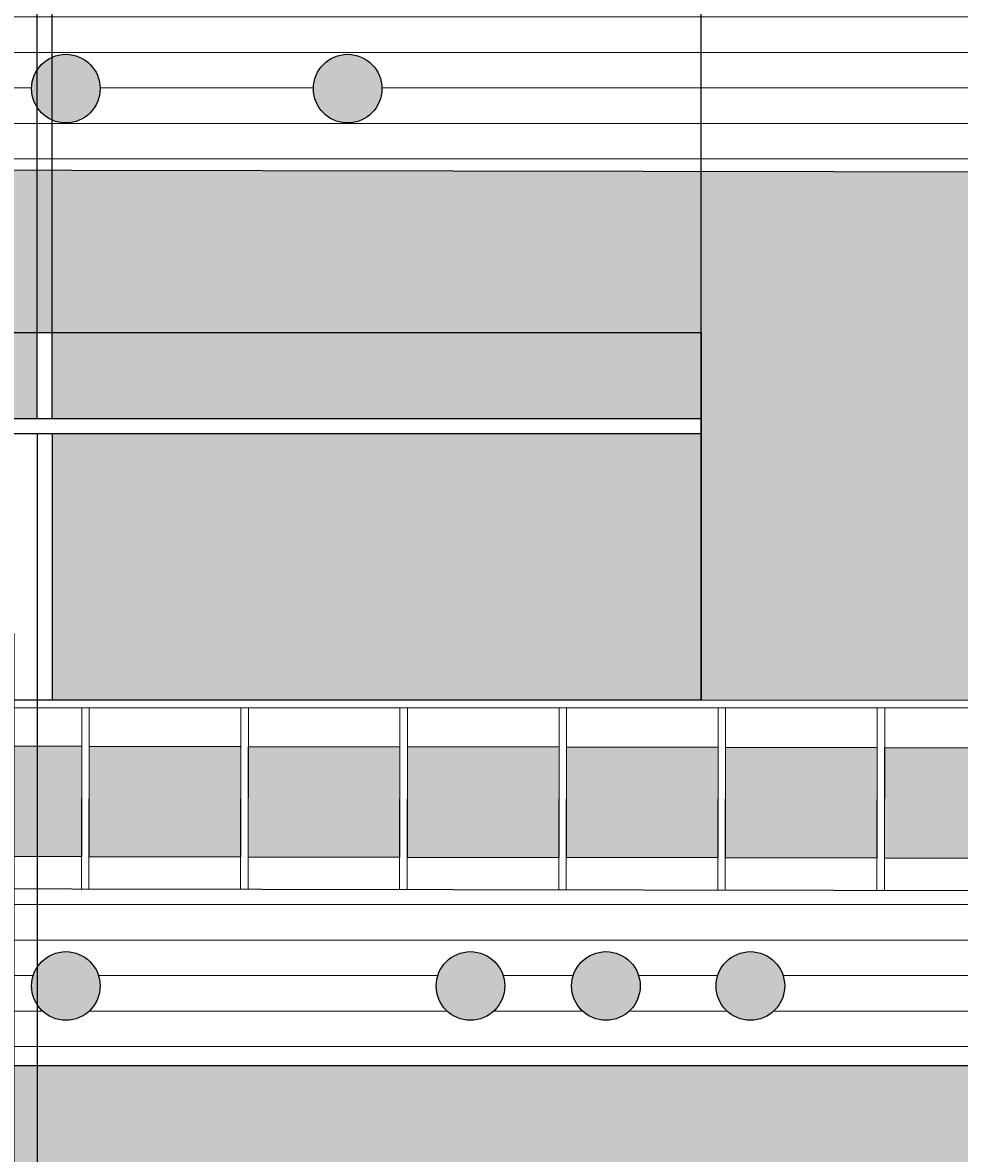
# Model space of a CAD drawing. Units: inches. Extents: x 36 to 594, y 79 to 831.
# Tile 10 of 30: x 265 to 390, y 294 to 446. Entities that reach past the tile are written whole.
import ezdxf

# ---------------------------------------------------------------- set-up
doc = ezdxf.new("R2010")
doc.units = ezdxf.units.IN
doc.header["$MEASUREMENT"] = 0
for name, color, linetype, lineweight in [('A-ANNO-DIMS', 2, 'Continuous', 18), ('A-ELEV', 7, 'Continuous', 25), ('A-ELEV-PATT', 8, 'Continuous', 13), ('A-GLAZ', 4, 'Continuous', 18)]:
    doc.layers.add(name, color=color, linetype=linetype, lineweight=lineweight)
doc.styles.get("Standard").update_dxf_attribs({"font": 'arial.ttf'})
doc.dimstyles.get("Standard").update_dxf_attribs({"dimtxt": 0.8125, "dimasz": 0.18, "dimexe": 0.18, "dimexo": 0.0625, "dimgap": 0.09, "dimtad": 0, "dimtih": 1, "dimtoh": 1, "dimdec": 4, "dimzin": 0, "dimdsep": 46, "dimlunit": 4, "dimtxsty": 'Standard', "dimcen": 0.09, "dimadec": 0, "dimazin": 0, "dimtfac": 1, "dimtdec": 4, "dimtofl": 0, "dimtmove": 0, "dimatfit": 3, "dimfxl": 1, "dimtolj": 1, "dimtzin": 0, "dimarcsym": 0})

# ---------------------------------------------------------------- blocks, each defined once
blk = doc.blocks.new('GLAZ-PANEL')
blk.add_lwpolyline([(0, 14.77), (20.28, 14.77), (20.28, 0), (0, 0)], close=True)
blk = doc.blocks.new('*D28')
at = {"layer": 'A-ANNO-DIMS', "color": 0, "lineweight": -2, "transparency": 16777216}
for p, q in [((269.3, 796.05), (37.49, 796.05)), ((37.67, 795.87), (37.67, 455.63)), ((37.67, 114.39), (37.67, 454.62)), ((94.8, 114.21), (37.49, 114.21))]:
    blk.add_line(p, q, dxfattribs=at)
at = {"layer": 'A-ANNO-DIMS', "color": 0, "transparency": 16777216}
for points in [[(37.64, 795.87), (37.7, 795.87), (37.67, 796.05)], [(37.64, 114.39), (37.7, 114.39), (37.67, 114.21)]]:
    blk.add_solid(points, dxfattribs=at)
at = {"layer": 'Defpoints', "color": 0, "transparency": 16777216}
for p in [(37.67, 796.05), (269.36, 796.05), (94.87, 114.21)]:
    blk.add_point(p, dxfattribs=at)
at = {"layer": 'A-ANNO-DIMS', "color": 0, "transparency": 16777216, "insert": (37.67, 455.13), "char_height": 0.812, "attachment_point": 5}
blk.add_mtext('\\A1;681.8', dxfattribs=at)
blk = doc.blocks.new('*D59')
at = {"layer": 'A-ANNO-DIMS', "color": 0, "lineweight": -2, "transparency": 16777216}
for p, q in [((355.86, 355.15), (355.86, 830.73)), ((356.04, 830.55), (388.74, 830.55)), ((424.37, 830.55), (391.67, 830.55)), ((424.55, 355.15), (424.55, 830.73))]:
    blk.add_line(p, q, dxfattribs=at)
at = {"layer": 'A-ANNO-DIMS', "color": 0, "transparency": 16777216}
for points in [[(356.04, 830.58), (356.04, 830.52), (355.86, 830.55)], [(424.37, 830.58), (424.37, 830.52), (424.55, 830.55)]]:
    blk.add_solid(points, dxfattribs=at)
at = {"layer": 'Defpoints', "color": 0, "transparency": 16777216}
for p in [(424.55, 830.55), (355.86, 355.08), (424.55, 355.08)]:
    blk.add_point(p, dxfattribs=at)
at = {"layer": 'A-ANNO-DIMS', "color": 0, "transparency": 16777216, "insert": (390.2, 830.55), "char_height": 0.812, "attachment_point": 5}
blk.add_mtext('\\A1;68.69', dxfattribs=at)
blk = doc.blocks.new('*D105')
at = {"layer": 'A-ANNO-DIMS', "color": 0, "lineweight": -2, "transparency": 16777216}
for p, q in [((241.36, 404.34), (241.36, 830.73)), ((241.54, 830.55), (252.42, 830.55)), ((266.86, 830.55), (255.98, 830.55)), ((267.04, 404.34), (267.04, 830.73))]:
    blk.add_line(p, q, dxfattribs=at)
at = {"layer": 'A-ANNO-DIMS', "color": 0, "transparency": 16777216}
for points in [[(241.54, 830.58), (241.54, 830.52), (241.36, 830.55)], [(266.86, 830.58), (266.86, 830.52), (267.04, 830.55)]]:
    blk.add_solid(points, dxfattribs=at)
at = {"layer": 'Defpoints', "color": 0, "transparency": 16777216}
for p in [(267.04, 830.55), (241.36, 404.27), (267.04, 404.27)]:
    blk.add_point(p, dxfattribs=at)
at = {"layer": 'A-ANNO-DIMS', "color": 0, "transparency": 16777216, "insert": (254.2, 830.55), "char_height": 0.812, "attachment_point": 5}
blk.add_mtext('\\A1;25.684', dxfattribs=at)
blk = doc.blocks.new('*D106')
at = {"layer": 'A-ANNO-DIMS', "color": 0, "lineweight": -2, "transparency": 16777216}
for p, q in [((267.04, 404.34), (267.04, 830.73)), ((267.22, 830.55), (267.68, 830.55)), ((268.86, 830.55), (268.4, 830.55)), ((269.04, 404.34), (269.04, 830.73))]:
    blk.add_line(p, q, dxfattribs=at)
at = {"layer": 'A-ANNO-DIMS', "color": 0, "transparency": 16777216}
for points in [[(267.22, 830.58), (267.22, 830.52), (267.04, 830.55)], [(268.86, 830.58), (268.86, 830.52), (269.04, 830.55)]]:
    blk.add_solid(points, dxfattribs=at)
at = {"layer": 'Defpoints', "color": 0, "transparency": 16777216}
for p in [(269.04, 830.55), (267.04, 404.27), (269.04, 404.27)]:
    blk.add_point(p, dxfattribs=at)
at = {"layer": 'A-ANNO-DIMS', "color": 0, "transparency": 16777216, "insert": (268.04, 830.55), "char_height": 0.812, "attachment_point": 5}
blk.add_mtext('\\A1;2', dxfattribs=at)
blk = doc.blocks.new('*D107')
at = {"layer": 'A-ANNO-DIMS', "color": 0, "lineweight": -2, "transparency": 16777216}
for p, q in [((269.04, 404.34), (269.04, 830.73)), ((269.22, 830.55), (310.99, 830.55)), ((355.68, 830.55), (313.91, 830.55)), ((355.86, 404.34), (355.86, 830.73))]:
    blk.add_line(p, q, dxfattribs=at)
at = {"layer": 'A-ANNO-DIMS', "color": 0, "transparency": 16777216}
for points in [[(269.22, 830.58), (269.22, 830.52), (269.04, 830.55)], [(355.68, 830.58), (355.68, 830.52), (355.86, 830.55)]]:
    blk.add_solid(points, dxfattribs=at)
at = {"layer": 'Defpoints', "color": 0, "transparency": 16777216}
for p in [(355.86, 830.55), (269.04, 404.27), (355.86, 404.27)]:
    blk.add_point(p, dxfattribs=at)
at = {"layer": 'A-ANNO-DIMS', "color": 0, "transparency": 16777216, "insert": (312.45, 830.55), "char_height": 0.812, "attachment_point": 5}
blk.add_mtext('\\A1;86.82', dxfattribs=at)
blk = doc.blocks.new('*D110')
at = {"layer": 'A-ANNO-DIMS', "color": 0, "lineweight": -2, "transparency": 16777216}
for p, q in [((263.89, 364.03), (263.89, 79.53)), ((267.04, 355.02), (267.04, 79.53)), ((264.07, 79.71), (264.32, 79.71)), ((266.86, 79.71), (266.61, 79.71))]:
    blk.add_line(p, q, dxfattribs=at)
at = {"layer": 'A-ANNO-DIMS', "color": 0, "transparency": 16777216}
for points in [[(264.07, 79.74), (264.07, 79.68), (263.89, 79.71)], [(266.86, 79.74), (266.86, 79.68), (267.04, 79.71)]]:
    blk.add_solid(points, dxfattribs=at)
at = {"layer": 'Defpoints', "color": 0, "transparency": 16777216}
for p in [(263.89, 364.09), (267.04, 355.08), (267.04, 79.71)]:
    blk.add_point(p, dxfattribs=at)
at = {"layer": 'A-ANNO-DIMS', "color": 0, "transparency": 16777216, "insert": (265.46, 79.71), "char_height": 0.812, "attachment_point": 5}
blk.add_mtext('\\A1;3.15', dxfattribs=at)

msp = doc.modelspace()

# ---------------------------------------------------------------- hatches: boundary and pattern name
at = {"layer": 'A-ELEV-PATT'}
h = msp.add_hatch(color=256, dxfattribs=at)
h.dxf.hatch_style = 1
h.paths.add_polyline_path([(398.0873, 796.0465), (269.3592, 796.0465), (269.3592, 770.1455), (397.8159, 770.1455)])
h.paths.add_polyline_path([(397.7518, 764.0341), (269.3592, 764.0341), (269.3592, 630.0394), (341.8367, 630.0394), (341.8367, 720.595), (335.0881, 728.3699), (329.982, 735.3373), (345.3661, 727.7743), (397.1052, 702.3389)])
h.paths.add_polyline_path([(341.8367, 594.2124), (201.4189, 594.2124), (201.4189, 475.4136), (232.8216, 475.4136), (232.8216, 524.6037), (341.8367, 524.6037)])
h.paths.add_polyline_path([(177.525, 594.2124), (118.7598, 594.2124), (118.7598, 450.2124), (177.525, 450.2124)])
h.paths.add_polyline_path([(424.4958, 594.2124), (365.7306, 594.2124), (365.7306, 450.2124), (424.4958, 450.2124)])
h.paths.add_polyline_path([(241.3553, 404.2737), (355.8569, 404.2737), (355.8569, 355.0836), (424.5492, 355.0836), (424.5492, 425.7333), (118.7598, 426.2844), (118.7598, 355.0836), (241.3553, 355.0836)])
h.paths.add_polyline_path([(448.3898, 306.2124), (217.0273, 306.2124), (217.0273, 142.2124), (254.0293, 142.2124), (254.0293, 150.9347), (254.0293, 286.1802), (401.5491, 286.1802), (401.5491, 150.9347), (401.5491, 142.2124), (448.3898, 142.2124)])
h.paths.add_polyline_path([(448.3898, 142.2124), (401.5491, 142.2124), (217.0273, 142.2124), (217.0273, 114.2124), (448.3898, 114.2124)])
h.paths.add_polyline_path([(217.0273, 306.2124), (174.7353, 306.2124), (94.8658, 306.2124), (94.8658, 162.2124), (103.3368, 162.2124), (103.3368, 264.6224), (103.3368, 286.1802), (217.0273, 286.1802)])
h = msp.add_hatch(color=256, dxfattribs=at)
h.dxf.hatch_style = 1
h.set_gradient(color1=(0, 255, 255), color2=(16, 86, 137))
h.paths.add_polyline_path([(341.8367, 524.6037), (260.5056, 524.6037), (260.5056, 513.1224), (341.8367, 513.1224)])
h.paths.add_polyline_path([(341.8367, 511.1224), (260.5056, 511.1224), (260.5056, 475.4136), (341.8367, 475.4136)])
h.paths.add_polyline_path([(258.5056, 524.6037), (232.8216, 524.6037), (232.8216, 513.1224), (258.5056, 513.1224)])
h.paths.add_polyline_path([(355.8569, 404.2737), (269.0393, 404.2737), (269.0393, 392.7924), (355.8569, 392.7924)])
h.paths.add_polyline_path([(267.0393, 404.2737), (241.3553, 404.2737), (241.3553, 392.7924), (267.0393, 392.7924)])
h.paths.add_polyline_path([(355.8569, 390.7924), (269.0393, 390.7924), (269.0393, 355.0836), (355.8569, 355.0836)])
h.paths.add_polyline_path([(399.5491, 284.1802), (256.0293, 284.1802), (256.0293, 271.378), (399.5491, 271.378)])
h.paths.add_polyline_path([(317.3533, 259.1243), (262.3169, 259.1243), (262.3169, 200.6645), (317.3533, 200.6645)])
h.paths.add_polyline_path([(390.386, 259.1243), (335.3496, 259.1243), (335.3496, 200.6645), (390.386, 200.6645)])
h.paths.add_polyline_path([(390.386, 190.7697), (335.3496, 190.7697), (335.3496, 162.9881), (390.386, 162.9881)])
h.paths.add_polyline_path([(317.3533, 190.7697), (262.3169, 190.7697), (262.3169, 162.9881), (317.3533, 162.9881)])
h.paths.add_polyline_path([(215.0273, 262.6224), (158.4069, 262.6224), (158.4069, 181.4195), (215.0273, 181.4195)])
h.paths.add_polyline_path([(215.0273, 284.1802), (105.3368, 284.1802), (105.3368, 266.6224), (215.0273, 266.6224)])
h = msp.add_hatch(color=256, dxfattribs=at)
h.dxf.hatch_style = 1
h.set_gradient(color1=(192, 192, 192), color2=(0, 0, 0))
h.paths.add_polyline_path([(243.19, 469.3251), (222.9132, 469.3251), (222.9132, 454.5571), (243.1634, 454.5571)])
h.paths.add_polyline_path([(264.4667, 469.2868), (244.1899, 469.2868), (244.1899, 454.5188), (264.4401, 454.5188)])
h.paths.add_polyline_path([(285.7435, 469.2484), (265.4667, 469.2484), (265.4667, 454.4804), (285.7168, 454.4804)])
h.paths.add_polyline_path([(307.0202, 469.2101), (286.7434, 469.2101), (286.7434, 454.4421), (306.9936, 454.4421)])
h.paths.add_polyline_path([(328.2969, 469.1717), (308.0201, 469.1717), (308.0201, 454.4037), (328.2703, 454.4037)])
h.paths.add_polyline_path([(341.8367, 469.1334), (329.2969, 469.1334), (329.2969, 454.3654), (341.8367, 454.3654)])
h.paths.add_polyline_path([(221.9133, 469.3635), (201.6365, 469.3635), (201.6365, 454.5955), (221.8866, 454.5955)])
h.paths.add_polyline_path([(145.3401, 349.1868), (125.0633, 349.1868), (125.0633, 334.4189), (145.3134, 334.4189)])
h.paths.add_polyline_path([(166.6168, 349.1485), (146.34, 349.1485), (146.34, 334.3805), (166.5902, 334.3805)])
h.paths.add_polyline_path([(187.8935, 349.1101), (167.6167, 349.1101), (167.6167, 334.3422), (187.8669, 334.3422)])
h.paths.add_polyline_path([(209.1703, 349.0718), (188.8935, 349.0718), (188.8935, 334.3038), (209.1436, 334.3038)])
h.paths.add_polyline_path([(230.447, 349.0335), (210.1702, 349.0335), (210.1702, 334.2655), (230.4204, 334.2655)])
h.paths.add_polyline_path([(251.7237, 348.9951), (231.4469, 348.9951), (231.4469, 334.2271), (251.6971, 334.2271)])
h.paths.add_polyline_path([(273.0005, 348.9568), (252.7236, 348.9568), (252.7236, 334.1888), (272.9738, 334.1888)])
h.paths.add_polyline_path([(294.2772, 348.9184), (274.0004, 348.9184), (274.0004, 334.1504), (294.2506, 334.1504)])
h.paths.add_polyline_path([(315.5539, 348.8801), (295.2771, 348.8801), (295.2771, 334.1121), (315.5273, 334.1121)])
h.paths.add_polyline_path([(336.8306, 348.8417), (316.5538, 348.8417), (316.5538, 334.0737), (336.804, 334.0737)])
h.paths.add_polyline_path([(358.1074, 348.8034), (337.8306, 348.8034), (337.8306, 334.0354), (358.0808, 334.0354)])
h.paths.add_polyline_path([(379.3841, 348.765), (359.1073, 348.765), (359.1073, 333.997), (379.3575, 333.997)])
h.paths.add_polyline_path([(400.6608, 348.7267), (380.384, 348.7267), (380.384, 333.9587), (400.6342, 333.9587)])
h.paths.add_polyline_path([(421.9376, 348.6883), (401.6608, 348.6883), (401.6608, 333.9204), (421.911, 333.9204)])
h.paths.add_polyline_path([(103.3368, 162.2124), (94.8658, 162.2124), (94.8658, 150.2124), (94.8658, 114.2124), (103.3368, 114.2124)])
h.paths.add_polyline_path([(217.0273, 132.2124), (103.3368, 132.2124), (103.3368, 122.2124), (217.0273, 122.2124)])
h.paths.add_polyline_path([(217.0273, 122.2124), (103.3368, 122.2124), (103.3368, 114.2124), (217.0273, 114.2124)])
h.paths.add_polyline_path([(217.0273, 142.2124), (174.7353, 142.2124), (103.3368, 142.2124), (103.3368, 132.2124), (217.0273, 132.2124)])
h.paths.add_polyline_path([(217.0273, 152.2124), (103.3368, 152.2124), (103.3368, 142.2124), (174.7353, 142.2124), (217.0273, 142.2124)])
h.paths.add_polyline_path([(217.0273, 162.2124), (103.3368, 162.2124), (103.3368, 152.2124), (217.0273, 152.2124)])
h = msp.add_hatch(dxfattribs=at)
h.set_pattern_fill('ANSI31', color=256, scale=38, angle=135)
h.paths.add_polyline_path([(448.3898, 450.2124), (94.8658, 450.2124), (94.8658, 306.2124), (174.7353, 306.2124), (448.3898, 306.2124), (448.3898, 367.5118)])
h.paths.add_polyline_path([(424.5492, 425.7333), (424.5492, 329.5325), (118.7598, 330.0836), (118.7598, 354.0836), (118.7598, 426.2844)], flags=16)
h.paths.add_polyline_path([(355.8569, 404.2737), (355.8569, 355.0836), (241.3553, 355.0836), (241.3553, 404.2737)], flags=0)
h.paths.add_polyline_path([(269.0393, 390.7924), (269.0393, 355.0836), (244.8248, 355.0836), (244.8248, 364.0887), (263.8892, 364.0887), (263.8892, 355.0836), (267.0393, 355.0836), (267.0393, 390.7924)], flags=0)
h.paths.add_polyline_path([(303.9765, 436.9126, -1), (313.1496, 436.9126, -1)], flags=16)
h.paths.add_polyline_path([(421.9473, 354.0836), (421.9376, 348.6883), (421.9376, 333.9204), (401.6342, 333.9204), (401.6705, 354.0836), (400.6705, 354.0836), (400.6608, 348.7267), (400.6608, 333.9587), (380.3574, 333.9587), (380.3937, 354.0836), (379.3937, 354.0836), (379.3841, 348.765), (379.3841, 333.997), (359.0807, 333.997), (359.1169, 354.0836), (358.1169, 354.0836), (358.1074, 348.8034), (358.1074, 334.0354), (337.804, 334.0354), (337.8401, 354.0836), (336.8401, 354.0836), (336.8306, 348.8417), (336.8306, 334.0737), (316.5272, 334.0737), (316.5633, 354.0836), (315.5633, 354.0836), (315.5539, 348.8801), (315.5539, 334.1121), (295.2505, 334.1121), (295.2865, 354.0836), (294.2865, 354.0836), (294.2772, 348.9184), (294.2772, 334.1504), (273.9738, 334.1504), (274.0097, 354.0836), (273.0097, 354.0836), (273.0005, 348.9568), (273.0005, 334.1888), (252.697, 334.1888), (252.7329, 354.0836), (251.7329, 354.0836), (251.7237, 348.9951), (251.7237, 334.2271), (231.4203, 334.2271), (231.4561, 354.0836), (230.4561, 354.0836), (230.447, 349.0335), (230.447, 334.2655), (210.1436, 334.2655), (210.1793, 354.0836), (209.1793, 354.0836), (209.1703, 349.0718), (209.1703, 334.3038), (188.8668, 334.3038), (188.9025, 354.0836), (187.9025, 354.0836), (187.8935, 349.1101), (187.8935, 334.3422), (167.5901, 334.3422), (167.6257, 354.0836), (166.6257, 354.0836), (166.6168, 349.1485), (166.6168, 334.3805), (146.3134, 334.3805), (146.3489, 354.0836), (145.3489, 354.0836), (145.3401, 349.1868), (145.3401, 334.4189), (125.0366, 334.4189), (125.0721, 354.0836)], flags=0)
h.paths.add_polyline_path([(266.285, 436.9126, -1), (275.458, 436.9126, -1)], flags=16)
h.paths.add_polyline_path([(367.0204, 316.8739, -1), (357.8474, 316.8739, -1)], flags=16)
h.paths.add_polyline_path([(347.6933, 316.8739, -1), (338.5202, 316.8739, -1)], flags=16)
h.paths.add_polyline_path([(329.574, 316.8739, -1), (320.401, 316.8739, -1)], flags=16)
h.paths.add_polyline_path([(263.8892, 385.1199), (263.8892, 368.1628), (244.8248, 368.1628), (244.8248, 385.1199)], flags=0)
h.paths.add_polyline_path([(216.2543, 436.9126, -1), (225.4274, 436.9126, -1)], flags=16)
h.paths.add_polyline_path([(275.458, 316.8739, -1), (266.285, 316.8739, -1)], flags=16)
h.paths.add_polyline_path([(225.4274, 316.8739, -1), (216.2543, 316.8739, -1)], flags=16)
h = msp.add_hatch(color=256, dxfattribs=at)
h.dxf.hatch_style = 1
h.paths.add_polyline_path([(313.1496, 436.9126, 1), (303.9765, 436.9126, 1)])
h.paths.add_polyline_path([(266.285, 436.9126, 1), (275.458, 436.9126, 1)])
h.paths.add_polyline_path([(225.4274, 436.9126, 1), (216.2543, 436.9126, 1)])
h.paths.add_polyline_path([(329.574, 316.8739, 1), (320.401, 316.8739, 1)])
h.paths.add_polyline_path([(347.6933, 316.8739, 1), (338.5202, 316.8739, 1)])
h.paths.add_polyline_path([(357.8474, 316.8739, 1), (367.0204, 316.8739, 1)])
h.paths.add_polyline_path([(275.458, 316.8739, 1), (266.285, 316.8739, 1)])
h.paths.add_polyline_path([(216.2543, 316.8739, 1), (225.4274, 316.8739, 1)])

# ---------------------------------------------------------------- linework, layer by layer
at = {"layer": 'A-ELEV'}
for p, q in [((267.0393, 392.7924), (267.0393, 404.2737)), ((269.0393, 392.7924), (269.0393, 404.2737)), ((241.3553, 392.7924), (355.8569, 392.7924)), ((241.3553, 390.7924), (355.8569, 390.7924)), ((267.0393, 390.7924), (267.0393, 355.0836)), ((269.0393, 390.7924), (269.0393, 355.0836)), ((174.7353, 306.2124), (448.3898, 306.2124))]:
    msp.add_line(p, q, dxfattribs=at)
for points in [[(118.7598, 426.2844), (424.5492, 425.7333), (424.5492, 329.5325), (118.7598, 330.0836)], [(241.3553, 404.2737), (355.8569, 404.2737), (355.8569, 355.0836), (241.3553, 355.0836)]]:
    msp.add_lwpolyline(points, close=True, dxfattribs=at)
for centre in [(270.8715, 436.9126), (308.5631, 436.9126), (270.8715, 316.8739), (324.9875, 316.8739), (343.1067, 316.8739), (362.4339, 316.8739)]:
    msp.add_circle(centre, 4.5865, dxfattribs=at)
at = {"layer": 'A-GLAZ'}
for p, q in [((118.7598, 355.0836), (424.5492, 355.0836)), ((118.7598, 354.0836), (424.5492, 354.0836)), ((273.0097, 354.0836), (272.966, 329.844)), ((274.0097, 354.0836), (273.966, 329.8422)), ((294.2865, 354.0836), (294.2427, 329.8057)), ((295.2865, 354.0836), (295.2427, 329.8039)), ((315.5633, 354.0836), (315.5195, 329.7673)), ((316.5633, 354.0836), (316.5195, 329.7655)), ((336.8401, 354.0836), (336.7962, 329.729)), ((337.8401, 354.0836), (337.7962, 329.7272)), ((358.1169, 354.0836), (358.0729, 329.6906)), ((359.1169, 354.0836), (359.0729, 329.6888)), ((379.3937, 354.0836), (379.3497, 329.6523)), ((380.3937, 354.0836), (380.3497, 329.6505))]:
    msp.add_line(p, q, dxfattribs=at)

# ---------------------------------------------------------------- block references
for p in [(252.7234, 334.1889), (274.0001, 334.1506), (295.2769, 334.1122), (316.5536, 334.0739), (337.8303, 334.0355), (359.1071, 333.9972), (380.3838, 333.9588)]:
    msp.add_blockref('GLAZ-PANEL', p, dxfattribs=at)

# ---------------------------------------------------------------- dimensions: what is measured, and where the dimension line sits
at = {"layer": 'A-ANNO-DIMS'}
for base, p1, p2, override, picture, middle in [((267.0393, 830.5465), (241.3553, 404.2737), (267.0393, 404.2737), {"dimdec": 3, "dimlfac": 1, "dimrnd": 0, "dimzin": 0, "dimdsep": 46, "dimlunit": 2}, '*D105', (254.1973, 830.5465)), ((269.0393, 830.5465), (267.0393, 404.2737), (269.0393, 404.2737), {"dimdec": 0, "dimlfac": 1, "dimrnd": 0, "dimzin": 0, "dimdsep": 46, "dimlunit": 2}, '*D106', (268.0393, 830.5465)), ((355.8569, 830.5465), (269.0393, 404.2737), (355.8569, 404.2737), {"dimdec": 2, "dimlfac": 1, "dimrnd": 0, "dimzin": 0, "dimdsep": 46, "dimlunit": 2}, '*D107', (312.4481, 830.5465)), ((424.5492, 830.5465), (355.8569, 355.0836), (424.5492, 355.0836), {"dimdec": 2, "dimlfac": 1, "dimrnd": 0, "dimzin": 0, "dimdsep": 46, "dimlunit": 2}, '*D59', (390.203, 830.5465)), ((267.0393, 79.7124), (263.8892, 364.0887), (267.0393, 355.0836), {"dimdec": 2, "dimlfac": 1, "dimrnd": 0, "dimzin": 0, "dimdsep": 46, "dimlunit": 2}, '*D110', (265.4643, 79.7124))]:
    dim = msp.add_linear_dim(base=base, p1=p1, p2=p2, dimstyle='Standard', override=override, dxfattribs=at)
    dim.commit()
    dim.dimension.update_dxf_attribs({"geometry": picture, "text_midpoint": middle})
dim = msp.add_linear_dim(base=(37.6733, 796.0465), p1=(94.8658, 114.2124), p2=(269.3592, 796.0465), angle=90, dimstyle='Standard', override={"dimdec": 1, "dimlfac": 1, "dimrnd": 0, "dimzin": 0, "dimdsep": 46, "dimlunit": 2}, dxfattribs=at)
dim.commit()
dim.dimension.update_dxf_attribs({"geometry": '*D28', "text_midpoint": (37.6733, 455.1294)})

doc.saveas('drawing.dxf')
